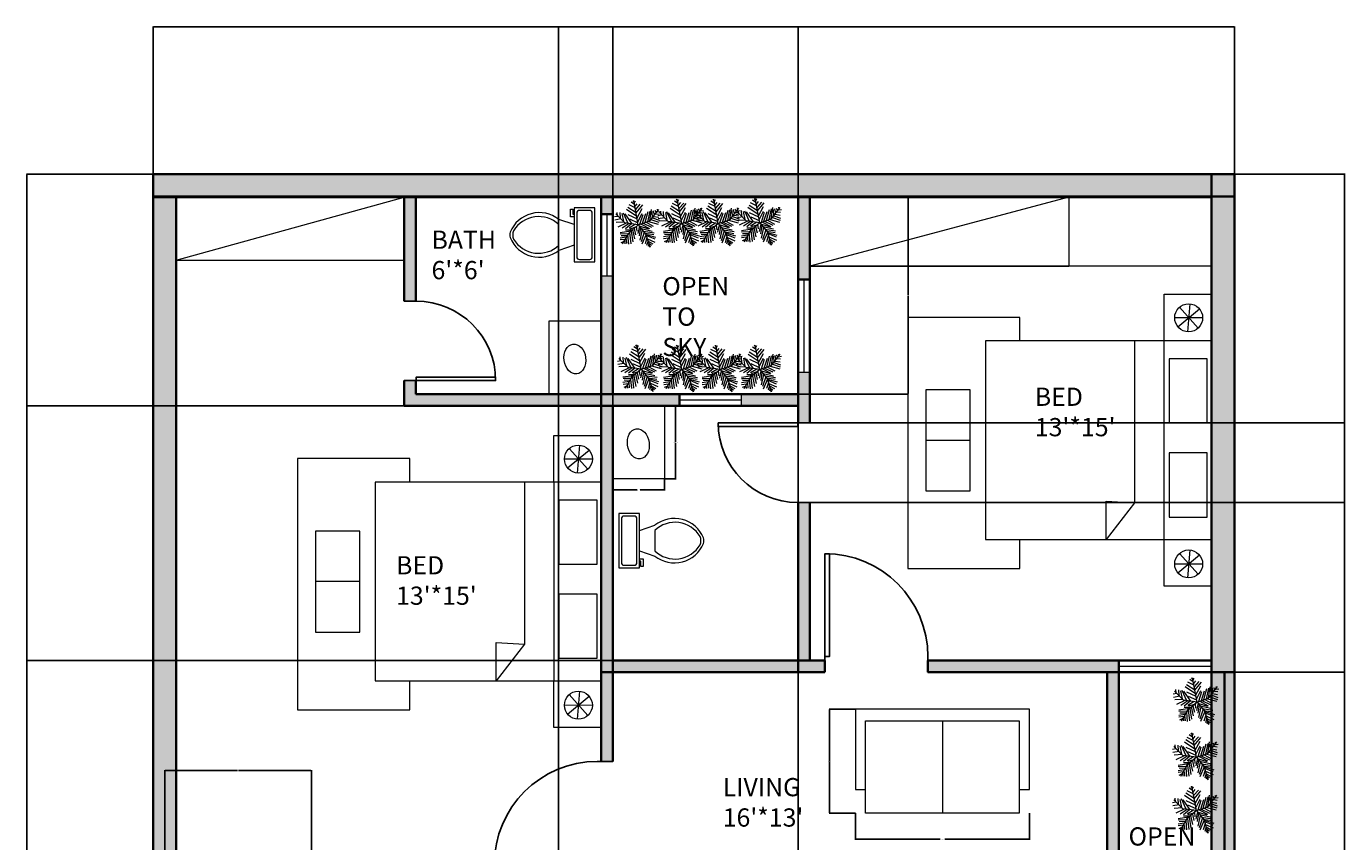
# Model space of a CAD drawing. Units: inches. Extents: x 2119 to 2631, y 2040 to 2935.
# Tile 3 of 3: x 2119 to 2631, y 2618 to 2935. Entities that reach past the tile are written whole.
import ezdxf

# ---------------------------------------------------------------- set-up
doc = ezdxf.new("R2010")
doc.units = ezdxf.units.IN
for name, color, linetype, lineweight in [('A-ANNO-DIMS', 2, 'Continuous', 18), ('A-AREA-IDEN', 7, 'Continuous', 18), ('A-FLOR-CASE', 33, 'Continuous', 18), ('A-FLOR-FIXT', 9, 'Continuous', 18), ('A-WALL-PATT', 252, 'Continuous', 13), ('C-PROP', 7, 'Continuous', 35), ('DOOR', 50, 'Continuous', 25), ('FURNITURE', 220, 'Continuous', 18), ('GRASS', 70, 'Continuous', 13), ('WALL', 180, 'Continuous', 35), ('WINDOW', 130, 'Continuous', 18)]:
    doc.layers.add(name, color=color, linetype=linetype, lineweight=lineweight)
doc.styles.get("Standard").update_dxf_attribs({"font": 'arial.ttf'})
doc.dimstyles.get("Standard").update_dxf_attribs({"dimtxt": 0.18, "dimasz": 0.18, "dimexe": 0.18, "dimexo": 0.0625, "dimgap": 0.09, "dimtad": 0, "dimtih": 1, "dimtoh": 1, "dimdec": 4, "dimzin": 0, "dimdsep": 46, "dimtxsty": 'Standard', "dimcen": 0.09, "dimadec": 0, "dimazin": 0, "dimtfac": 1, "dimtdec": 4, "dimtofl": 0, "dimtmove": 0, "dimatfit": 3, "dimfxl": 1, "dimtolj": 1, "dimtzin": 0, "dimarcsym": 0})

# ---------------------------------------------------------------- blocks, each defined once
blk = doc.blocks.new('*U2')
for p, q in [((0, 0), (0, -6)), ((40, 0), (40, -6))]:
    blk.add_line(p, q)
blk.add_lwpolyline([(0, 0), (0, 40), (1.75, 40), (1.75, 0)], close=True)
blk.add_arc((0, 0), 40, 0, 90)
blk = doc.blocks.new('*U4')
for p, q in [((9.5, -6), (9.5, -2)), ((-10, -8.5), (-8, -8.5)), ((-10, -9.5), (-10, -8.5)), ((-7, -9.5), (-10, -9.5)), ((-8, -8.5), (-8, -8)), ((-7, -8), (-7, -9.5)), ((-4, -8), (-6, -14)), ((4, -8), (6, -14)), ((4, -14), (-4, -14))]:
    blk.add_line(p, q)
blk.add_lwpolyline([(10.5, -8), (10.5, 0), (-10.5, 0), (-10.5, -8)], close=True)
for points in [[(-9.5, -2), (-9.5, -6)], [(8.5, -1), (-8.5, -1)], [(-8.5, -7), (8.5, -7)]]:
    blk.add_lwpolyline(points)
for centre, radius, start, end in [((-8.62, -1.88), 0.884, 81.8699, 188.1301), ((8.62, -1.88), 0.884, 351.8699, 98.1301), ((-8.62, -6.12), 0.884, 171.8699, 278.1301), ((8.62, -6.12), 0.884, 261.8699, 8.1301), ((3.52, -21.58), 12.17, 141.4691, 247.9714), ((4.2, -21.82), 11.33, 136.3677, 238.9468), ((-3.52, -21.58), 12.17, 292.0284, 38.5307), ((-4.2, -21.82), 11.33, 301.053, 43.6321), ((0, -27.88), 4, 245.7318, 294.2682), ((0, -29), 4, 254.8605, 285.1395)]:
    blk.add_arc(centre, radius, start, end)
blk = doc.blocks.new('*U6')
for p, q in [((-3.665, 19.273), (-27.574, 35.527)), ((-5.114, 28.097), (-24.676, 40.636)), ((-7.288, 39.707), (-21.778, 46.673)), ((-8.737, 47.138), (-17.069, 52.711)), ((-10.186, 53.64), (-13.084, 55.962)), ((0, 0), (-10.5, 57)), ((-9.099, 51.782), (-6.563, 55.962)), ((-7.65, 43.423), (-2.578, 49.46)), ((-5.839, 35.992), (4.667, 48.067)), ((-5.114, 27.632), (10.463, 46.673)), ((-2.941, 16.486), (8.652, 37.85)), ((16.259, 5.805), (23.142, 31.348)), ((22.055, 7.198), (27.489, 32.277)), ((27, 9), (48, 36)), ((27.127, 9.056), (31.112, 35.992)), ((35.096, 32.741), (37.27, 22.524)), ((38.719, 34.134), (41.979, 28.561)), ((44.153, 36.456), (45.239, 32.741)), ((-47.498, 19.737), (-55.83, 18.344)), ((-40.615, 13.7), (-55.105, 10.913)), ((-31.5, 4.5), (-52.5, 25.5)), ((-33.37, 6.269), (-52.207, 5.34)), ((-48.585, 21.131), (-49.309, 29.026)), ((-28.299, 3.483), (-47.86, -5.805)), ((-43.513, 28.561), (-42.427, 15.558)), ((-38.442, 26.239), (-34.819, 7.663)), ((-21.416, 3.018), (-38.079, -8.128)), ((-35.544, 28.097), (-24.314, 3.947)), ((0, 0), (-31.5, 4.5)), ((-14.533, 2.09), (-30.834, 25.31)), ((-15.982, 2.09), (-30.11, -9.521)), ((-24.314, 23.917), (-2.941, 13.7)), ((0, 0), (-22.5, -19.5)), ((-6.563, 1.161), (-21.416, -8.128)), ((-20.691, 13.7), (-1.129, 4.876)), ((-1.129, 6.734), (9.014, 26.704)), ((0, 0), (27, 9)), ((0, 0), (18, -22.5)), ((3.942, 1.625), (11.187, 24.381)), ((6.478, 1.625), (26.04, -8.592)), ((10.101, 3.483), (17.708, 26.239)), ((11.187, 3.483), (30.749, -5.805)), ((18.07, 5.805), (35.096, -3.483)), ((24.229, 7.663), (46.688, 1.625)), ((29.662, 12.307), (48.137, 6.269)), ((31.836, 30.883), (32.561, 16.486)), ((33.285, 16.486), (48.862, 10.913)), ((36.183, 19.737), (48.137, 17.88)), ((40.53, 25.775), (48.862, 24.846)), ((43.791, 29.954), (51.036, 30.883)), ((-17.431, -15.094), (-42.789, -18.809)), ((-28.299, -29.026), (-42.789, -31.348)), ((-24.314, -21.596), (-42.427, -22.06)), ((-26.849, -26.24), (-40.253, -25.775)), ((-22.5, -19.5), (-37.5, -45)), ((-15.257, -12.772), (-30.11, -12.772)), ((-29.023, -30.884), (-27.936, -43.887)), ((-25.038, -23.918), (-22.865, -45.281)), ((-20.691, -18.345), (-17.793, -44.352)), ((-6.563, -5.805), (-19.967, -9.985)), ((-17.069, -15.094), (-12.721, -40.172)), ((-13.446, -11.378), (-8.737, -32.741)), ((-9.461, -8.592), (-6.201, -23.453)), ((-4.752, -3.483), (-3.665, -14.629)), ((2.493, -3.019), (-1.491, -20.202)), ((1.769, -2.555), (24.229, -9.521)), ((5.029, -6.27), (2.131, -25.775)), ((9.014, -11.378), (3.58, -35.992)), ((14.085, -16.951), (6.478, -40.172)), ((7.565, -9.056), (32.198, -14.629)), ((18.07, -22.524), (8.289, -45.745)), ((12.274, -15.094), (36.907, -18.809)), ((20.244, -30.419), (15.897, -44.816)), ((16.259, -19.738), (36.183, -22.989)), ((18, -22.5), (27, -52.5)), ((18.433, -22.524), (40.53, -29.026)), ((19.157, -25.311), (38.719, -33.206)), ((-30.834, -34.135), (-42.427, -35.528)), ((-34.457, -39.708), (-40.978, -42.494)), ((-32.646, -36.921), (-31.921, -44.352)), ((22.78, -37.85), (19.519, -48.532)), ((21.331, -32.741), (39.081, -40.636)), ((22.78, -38.314), (34.372, -44.816)), ((24.591, -45.745), (23.142, -50.854)), ((24.591, -43.423), (30.749, -47.603)), ((26.764, -49.925), (28.213, -50.854))]:
    blk.add_line(p, q)
blk = doc.blocks.new('BED-DOUBLE-SUITE')
for p, q in [((-13.02, 5.47), (-4.66, 12.4)), ((-12.38, 13.04), (-5.14, 4.94)), ((-9.21, 3.5), (-8.22, 14.32)), ((-74.36, 9.08), (-117.92, 9.08)), ((-117.92, 9.08), (-117.92, -88.45)), ((-74.36, 0), (-74.36, 9.08)), ((-14.26, 9.02), (-3.4, 8.97)), ((-29.81, 0), (-29.81, -62.95)), ((-18.41, 0), (-18.41, -77.17)), ((-93.69, -38.69), (-110.95, -38.69)), ((-40.83, -77.17), (-40.83, -62.28)), ((-40.83, -62.28), (-29.81, -62.95)), ((-29.81, -62.95), (-40.83, -77.17)), ((-74.36, -88.45), (-74.36, -77.17)), ((-9.21, -92.12), (-8.22, -81.31)), ((-14.26, -86.6), (-3.4, -86.65)), ((-13.02, -90.15), (-4.66, -83.22)), ((-12.38, -82.59), (-5.14, -90.68)), ((-117.92, -88.45), (-74.36, -88.45))]:
    blk.add_line(p, q)
for points in [[(0, 0), (-18.39, 0), (-18.39, 18.13), (0, 18.13)], [(0, 0), (-87.71, 0), (-87.71, -77.17), (0, -77.17)], [(-1.58, -7.03), (-16.39, -7.03), (-16.39, -31.92), (-1.58, -31.92)], [(-93.69, -19.1), (-110.95, -19.1), (-110.95, -58.28), (-93.69, -58.28)], [(-1.58, -43.58), (-16.39, -43.58), (-16.39, -68.47), (-1.58, -68.47)], [(0, -95.3), (-18.39, -95.3), (-18.39, -77.17), (0, -77.17)]]:
    blk.add_lwpolyline(points, close=True)
for centre in [(-8.83, 8.92), (-8.83, -86.7)]:
    blk.add_circle(centre, 5.43)
blk = doc.blocks.new('SOFA-2-SEAT')
for p, q in [((-9.19, 63.72), (-40.39, 63.72)), ((-40.39, 63.72), (-40.39, -3.87)), ((-9.19, 59.66), (-9.19, 63.72)), ((-35.92, 29.83), (0, 29.83)), ((-9.19, -3.87), (-9.19, 0)), ((-40.39, -3.87), (-9.19, -3.87))]:
    blk.add_line(p, q)
blk.add_lwpolyline([(0, 0), (-35.92, 0), (-35.92, 59.66), (0, 59.66)], close=True)
blk = doc.blocks.new('BASIN-VANITY')
blk.add_lwpolyline([(0, 0), (-20.15, 0), (-20.15, 28.46), (0, 28.46)], close=True)
blk.add_ellipse((-10.21, 13.63), major_axis=(0.77, -5.8), ratio=0.722636)
blk = doc.blocks.new('*D14')
at = {"layer": 'A-ANNO-DIMS', "color": 0, "lineweight": -2, "transparency": 16777216}
for p, q in [((2441.07, 2629.04), (2441.07, 2618.79)), ((2508.66, 2629.04), (2508.66, 2618.79)), ((2441.25, 2618.97), (2473.96, 2618.97)), ((2508.48, 2618.97), (2475.77, 2618.97))]:
    blk.add_line(p, q, dxfattribs=at)
at = {"layer": 'A-ANNO-DIMS', "color": 0, "lineweight": 100, "transparency": 16777216}
for points in [[(2441.25, 2619), (2441.25, 2618.94), (2441.07, 2618.97)], [(2508.48, 2619), (2508.48, 2618.94), (2508.66, 2618.97)]]:
    blk.add_solid(points, dxfattribs=at)
at = {"layer": 'Defpoints', "color": 0, "lineweight": 100, "transparency": 16777216}
for p in [(2441.07, 2629.11), (2508.66, 2629.11), (2508.66, 2618.97)]:
    blk.add_point(p, dxfattribs=at)
at = {"layer": 'A-ANNO-DIMS', "color": 0, "transparency": 16777216, "insert": (2474.87, 2618.97), "char_height": 0.18, "attachment_point": 5}
blk.add_mtext('\\A1;SOFA 68 TYP.', dxfattribs=at)
blk = doc.blocks.new('*D15')
at = {"layer": 'A-ANNO-DIMS', "color": 0, "lineweight": -2, "transparency": 16777216}
for p, q in [((2441.01, 2669.5), (2430.76, 2669.5)), ((2430.94, 2669.32), (2430.94, 2649.48)), ((2430.94, 2629.29), (2430.94, 2649.12)), ((2441.01, 2629.11), (2430.76, 2629.11))]:
    blk.add_line(p, q, dxfattribs=at)
at = {"layer": 'A-ANNO-DIMS', "color": 0, "lineweight": 100, "transparency": 16777216}
for points in [[(2430.91, 2669.32), (2430.97, 2669.32), (2430.94, 2669.5)], [(2430.91, 2629.29), (2430.97, 2629.29), (2430.94, 2629.11)]]:
    blk.add_solid(points, dxfattribs=at)
at = {"layer": 'Defpoints', "color": 0, "lineweight": 100, "transparency": 16777216}
for p in [(2441.07, 2669.5), (2430.94, 2629.11), (2441.07, 2629.11)]:
    blk.add_point(p, dxfattribs=at)
at = {"layer": 'A-ANNO-DIMS', "color": 0, "transparency": 16777216, "insert": (2430.94, 2649.3), "char_height": 0.18, "attachment_point": 5}
blk.add_mtext('\\A1;40 TYP.', dxfattribs=at)
blk = doc.blocks.new('*D16')
at = {"layer": 'A-ANNO-DIMS', "color": 0, "lineweight": -2, "transparency": 16777216}
for p, q in [((2366.96, 2787.4), (2371.35, 2787.4)), ((2371.17, 2787.22), (2371.17, 2773.35)), ((2371.17, 2759.12), (2371.17, 2772.99)), ((2366.96, 2758.94), (2371.35, 2758.94))]:
    blk.add_line(p, q, dxfattribs=at)
at = {"layer": 'A-ANNO-DIMS', "color": 0, "lineweight": 100, "transparency": 16777216}
for points in [[(2371.14, 2787.22), (2371.2, 2787.22), (2371.17, 2787.4)], [(2371.14, 2759.12), (2371.2, 2759.12), (2371.17, 2758.94)]]:
    blk.add_solid(points, dxfattribs=at)
at = {"layer": 'Defpoints', "color": 0, "lineweight": 100, "transparency": 16777216}
for p in [(2366.9, 2787.4), (2371.17, 2787.4), (2366.9, 2758.94)]:
    blk.add_point(p, dxfattribs=at)
at = {"layer": 'A-ANNO-DIMS', "color": 0, "transparency": 16777216, "insert": (2371.17, 2773.17), "char_height": 0.18, "attachment_point": 5}
blk.add_mtext('\\A1;VANITY 28 TYP.', dxfattribs=at)
blk = doc.blocks.new('*D17')
at = {"layer": 'A-ANNO-DIMS', "color": 0, "lineweight": -2, "transparency": 16777216}
for p, q in [((2346.75, 2758.88), (2346.75, 2754.49)), ((2366.9, 2758.88), (2366.9, 2754.49)), ((2346.93, 2754.67), (2356.3, 2754.67)), ((2366.72, 2754.67), (2357.36, 2754.67))]:
    blk.add_line(p, q, dxfattribs=at)
at = {"layer": 'A-ANNO-DIMS', "color": 0, "lineweight": 100, "transparency": 16777216}
for points in [[(2346.93, 2754.7), (2346.93, 2754.64), (2346.75, 2754.67)], [(2366.72, 2754.7), (2366.72, 2754.64), (2366.9, 2754.67)]]:
    blk.add_solid(points, dxfattribs=at)
at = {"layer": 'Defpoints', "color": 0, "lineweight": 100, "transparency": 16777216}
for p in [(2346.75, 2758.94), (2366.9, 2758.94), (2366.9, 2754.67)]:
    blk.add_point(p, dxfattribs=at)
at = {"layer": 'A-ANNO-DIMS', "color": 0, "transparency": 16777216, "insert": (2356.83, 2754.67), "char_height": 0.18, "attachment_point": 5}
blk.add_mtext('\\A1;20 TYP.', dxfattribs=at)
blk = doc.blocks.new('*D18')
at = {"layer": 'A-ANNO-DIMS', "color": 0, "lineweight": -2, "transparency": 16777216}
for p, q in [((2168.25, 2877.46), (2168.25, 2934.76)), ((2168.43, 2934.58), (2377.96, 2934.58)), ((2588.07, 2934.58), (2378.55, 2934.58)), ((2588.25, 2877.46), (2588.25, 2934.76))]:
    blk.add_line(p, q, dxfattribs=at)
at = {"layer": 'A-ANNO-DIMS', "color": 0, "lineweight": 100, "transparency": 16777216}
for points in [[(2168.43, 2934.61), (2168.43, 2934.55), (2168.25, 2934.58)], [(2588.07, 2934.61), (2588.07, 2934.55), (2588.25, 2934.58)]]:
    blk.add_solid(points, dxfattribs=at)
at = {"layer": 'Defpoints', "color": 0, "lineweight": 100, "transparency": 16777216}
for p in [(2588.25, 2934.58), (2168.25, 2877.4), (2588.25, 2877.4)]:
    blk.add_point(p, dxfattribs=at)
at = {"layer": 'A-ANNO-DIMS', "color": 0, "transparency": 16777216, "insert": (2378.25, 2934.58), "char_height": 0.18, "attachment_point": 5}
blk.add_mtext('\\A1;420', dxfattribs=at)
blk = doc.blocks.new('*D19')
at = {"layer": 'A-ANNO-DIMS', "color": 0, "lineweight": -2, "transparency": 16777216}
for p, q in [((2168.19, 2877.4), (2119.07, 2877.4)), ((2119.25, 2877.22), (2119.25, 2487.58)), ((2119.25, 2097.58), (2119.25, 2487.22)), ((2168.19, 2097.4), (2119.07, 2097.4))]:
    blk.add_line(p, q, dxfattribs=at)
at = {"layer": 'A-ANNO-DIMS', "color": 0, "lineweight": 100, "transparency": 16777216}
for points in [[(2119.22, 2877.22), (2119.28, 2877.22), (2119.25, 2877.4)], [(2119.22, 2097.58), (2119.28, 2097.58), (2119.25, 2097.4)]]:
    blk.add_solid(points, dxfattribs=at)
at = {"layer": 'Defpoints', "color": 0, "lineweight": 100, "transparency": 16777216}
for p in [(2119.25, 2877.4), (2168.25, 2877.4), (2168.25, 2097.4)]:
    blk.add_point(p, dxfattribs=at)
at = {"layer": 'A-ANNO-DIMS', "color": 0, "transparency": 16777216, "insert": (2119.25, 2487.4), "char_height": 0.18, "attachment_point": 5}
blk.add_mtext('\\A1;780', dxfattribs=at)
blk = doc.blocks.new('*D21')
at = {"layer": 'A-ANNO-DIMS', "color": 0, "lineweight": -2, "transparency": 16777216}
for p, q in [((2325.75, 2175.46), (2325.75, 2934.76)), ((2325.93, 2934.58), (2372.04, 2934.58)), ((2418.57, 2934.58), (2372.47, 2934.58)), ((2418.75, 2175.46), (2418.75, 2934.76))]:
    blk.add_line(p, q, dxfattribs=at)
at = {"layer": 'A-ANNO-DIMS', "color": 0, "lineweight": 100, "transparency": 16777216}
for points in [[(2325.93, 2934.61), (2325.93, 2934.55), (2325.75, 2934.58)], [(2418.57, 2934.61), (2418.57, 2934.55), (2418.75, 2934.58)]]:
    blk.add_solid(points, dxfattribs=at)
at = {"layer": 'Defpoints', "color": 0, "lineweight": 100, "transparency": 16777216}
for p in [(2418.75, 2934.58), (2325.75, 2175.4), (2418.75, 2175.4)]:
    blk.add_point(p, dxfattribs=at)
at = {"layer": 'A-ANNO-DIMS', "color": 0, "transparency": 16777216, "insert": (2372.25, 2934.58), "char_height": 0.18, "attachment_point": 5}
blk.add_mtext('\\A1;93', dxfattribs=at)
blk = doc.blocks.new('*D25')
at = {"layer": 'A-ANNO-DIMS', "color": 0, "lineweight": -2, "transparency": 16777216}
for p, q in [((2588.32, 2683.9), (2631.18, 2683.9)), ((2631, 2683.72), (2631, 2606.21)), ((2631, 2528.34), (2631, 2605.85)), ((2588.32, 2528.16), (2631.18, 2528.16))]:
    blk.add_line(p, q, dxfattribs=at)
at = {"layer": 'A-ANNO-DIMS', "color": 0, "lineweight": 100, "transparency": 16777216}
for points in [[(2630.97, 2683.72), (2631.03, 2683.72), (2631, 2683.9)], [(2630.97, 2528.34), (2631.03, 2528.34), (2631, 2528.16)]]:
    blk.add_solid(points, dxfattribs=at)
at = {"layer": 'Defpoints', "color": 0, "lineweight": 100, "transparency": 16777216}
for p in [(2588.25, 2683.9), (2631, 2683.9), (2588.25, 2528.16)]:
    blk.add_point(p, dxfattribs=at)
at = {"layer": 'A-ANNO-DIMS', "color": 0, "transparency": 16777216, "insert": (2631, 2606.03), "char_height": 0.18, "attachment_point": 5}
blk.add_mtext('\\A1;155.74', dxfattribs=at)
blk = doc.blocks.new('*D26')
at = {"layer": 'A-ANNO-DIMS', "color": 0, "lineweight": -2, "transparency": 16777216}
for p, q in [((2588.32, 2877.4), (2631.18, 2877.4)), ((2631, 2877.22), (2631, 2780.83)), ((2631, 2684.08), (2631, 2780.47)), ((2588.32, 2683.9), (2631.18, 2683.9))]:
    blk.add_line(p, q, dxfattribs=at)
at = {"layer": 'A-ANNO-DIMS', "color": 0, "lineweight": 100, "transparency": 16777216}
for points in [[(2630.97, 2877.22), (2631.03, 2877.22), (2631, 2877.4)], [(2630.97, 2684.08), (2631.03, 2684.08), (2631, 2683.9)]]:
    blk.add_solid(points, dxfattribs=at)
at = {"layer": 'Defpoints', "color": 0, "lineweight": 100, "transparency": 16777216}
for p in [(2588.25, 2877.4), (2631, 2877.4), (2588.25, 2683.9)]:
    blk.add_point(p, dxfattribs=at)
at = {"layer": 'A-ANNO-DIMS', "color": 0, "transparency": 16777216, "insert": (2631, 2780.65), "char_height": 0.18, "attachment_point": 5}
blk.add_mtext('\\A1;193.5', dxfattribs=at)
blk = doc.blocks.new('*D27')
at = {"layer": 'A-ANNO-DIMS', "color": 0, "lineweight": -2, "transparency": 16777216}
for p, q in [((2346.75, 2688.46), (2346.75, 2934.76)), ((2346.93, 2934.58), (2382.54, 2934.58)), ((2418.57, 2934.58), (2382.97, 2934.58)), ((2418.75, 2688.46), (2418.75, 2934.76))]:
    blk.add_line(p, q, dxfattribs=at)
at = {"layer": 'A-ANNO-DIMS', "color": 0, "lineweight": 100, "transparency": 16777216}
for points in [[(2346.93, 2934.61), (2346.93, 2934.55), (2346.75, 2934.58)], [(2418.57, 2934.61), (2418.57, 2934.55), (2418.75, 2934.58)]]:
    blk.add_solid(points, dxfattribs=at)
at = {"layer": 'Defpoints', "color": 0, "lineweight": 100, "transparency": 16777216}
for p in [(2418.75, 2934.58), (2346.75, 2688.4), (2418.75, 2688.4)]:
    blk.add_point(p, dxfattribs=at)
at = {"layer": 'A-ANNO-DIMS', "color": 0, "transparency": 16777216, "insert": (2382.75, 2934.58), "char_height": 0.18, "attachment_point": 5}
blk.add_mtext('\\A1;72', dxfattribs=at)
blk = doc.blocks.new('*D28')
at = {"layer": 'A-ANNO-DIMS', "color": 0, "lineweight": -2, "transparency": 16777216}
for p, q in [((2418.69, 2787.4), (2119.07, 2787.4)), ((2119.25, 2787.22), (2119.25, 2738.08)), ((2119.25, 2688.58), (2119.25, 2737.72)), ((2418.69, 2688.4), (2119.07, 2688.4))]:
    blk.add_line(p, q, dxfattribs=at)
at = {"layer": 'A-ANNO-DIMS', "color": 0, "lineweight": 100, "transparency": 16777216}
for points in [[(2119.22, 2787.22), (2119.28, 2787.22), (2119.25, 2787.4)], [(2119.22, 2688.58), (2119.28, 2688.58), (2119.25, 2688.4)]]:
    blk.add_solid(points, dxfattribs=at)
at = {"layer": 'Defpoints', "color": 0, "lineweight": 100, "transparency": 16777216}
for p in [(2119.25, 2787.4), (2418.75, 2787.4), (2418.75, 2688.4)]:
    blk.add_point(p, dxfattribs=at)
at = {"layer": 'A-ANNO-DIMS', "color": 0, "transparency": 16777216, "insert": (2119.25, 2737.9), "char_height": 0.18, "attachment_point": 5}
blk.add_mtext('\\A1;99', dxfattribs=at)
blk = doc.blocks.new('*D29')
at = {"layer": 'A-ANNO-DIMS', "color": 0, "lineweight": -2, "transparency": 16777216}
for p, q in [((2423.32, 2780.71), (2631.18, 2780.71)), ((2631, 2780.53), (2631, 2765.45)), ((2631, 2749.99), (2631, 2765.08)), ((2423.32, 2749.81), (2631.18, 2749.81))]:
    blk.add_line(p, q, dxfattribs=at)
at = {"layer": 'A-ANNO-DIMS', "color": 0, "lineweight": 100, "transparency": 16777216}
for points in [[(2630.97, 2780.53), (2631.03, 2780.53), (2631, 2780.71)], [(2630.97, 2749.99), (2631.03, 2749.99), (2631, 2749.81)]]:
    blk.add_solid(points, dxfattribs=at)
at = {"layer": 'Defpoints', "color": 0, "lineweight": 100, "transparency": 16777216}
for p in [(2423.25, 2780.71), (2631, 2780.71), (2423.25, 2749.81)]:
    blk.add_point(p, dxfattribs=at)
at = {"layer": 'A-ANNO-DIMS', "color": 0, "transparency": 16777216, "insert": (2631, 2765.26), "char_height": 0.18, "attachment_point": 5}
blk.add_mtext('\\A1;30.897', dxfattribs=at)
blk = doc.blocks.new('*D30')
at = {"layer": 'A-ANNO-DIMS', "color": 0, "lineweight": -2, "transparency": 16777216}
for p, q in [((2172.75, 2602.96), (2172.75, 2645.83)), ((2172.93, 2645.65), (2201.04, 2645.65)), ((2229.57, 2645.65), (2201.47, 2645.65)), ((2229.75, 2602.96), (2229.75, 2645.83))]:
    blk.add_line(p, q, dxfattribs=at)
at = {"layer": 'A-ANNO-DIMS', "color": 0, "lineweight": 100, "transparency": 16777216}
for points in [[(2172.93, 2645.68), (2172.93, 2645.62), (2172.75, 2645.65)], [(2229.57, 2645.68), (2229.57, 2645.62), (2229.75, 2645.65)]]:
    blk.add_solid(points, dxfattribs=at)
at = {"layer": 'Defpoints', "color": 0, "lineweight": 100, "transparency": 16777216}
for p in [(2229.75, 2645.65), (2172.75, 2602.9), (2229.75, 2602.9)]:
    blk.add_point(p, dxfattribs=at)
at = {"layer": 'A-ANNO-DIMS', "color": 0, "transparency": 16777216, "insert": (2201.25, 2645.65), "char_height": 0.18, "attachment_point": 5}
blk.add_mtext('\\A1;57', dxfattribs=at)
blk = doc.blocks.new('*D31')
at = {"layer": 'A-ANNO-DIMS', "color": 0, "lineweight": -2, "transparency": 16777216}
for p, q in [((2543.25, 2683.84), (2543.25, 2054.47)), ((2579.25, 2683.84), (2579.25, 2054.47)), ((2543.43, 2054.65), (2561.04, 2054.65)), ((2579.07, 2054.65), (2561.47, 2054.65))]:
    blk.add_line(p, q, dxfattribs=at)
at = {"layer": 'A-ANNO-DIMS', "color": 0, "lineweight": 100, "transparency": 16777216}
for points in [[(2543.43, 2054.68), (2543.43, 2054.62), (2543.25, 2054.65)], [(2579.07, 2054.68), (2579.07, 2054.62), (2579.25, 2054.65)]]:
    blk.add_solid(points, dxfattribs=at)
at = {"layer": 'Defpoints', "color": 0, "lineweight": 100, "transparency": 16777216}
for p in [(2543.25, 2683.9), (2579.25, 2683.9), (2579.25, 2054.65)]:
    blk.add_point(p, dxfattribs=at)
at = {"layer": 'A-ANNO-DIMS', "color": 0, "transparency": 16777216, "insert": (2561.25, 2054.65), "char_height": 0.18, "attachment_point": 5}
blk.add_mtext('\\A1;36', dxfattribs=at)
blk = doc.blocks.new('*D32')
at = {"layer": 'A-ANNO-DIMS', "color": 0, "lineweight": -2, "transparency": 16777216}
for p, q in [((2418.82, 2868.4), (2461.68, 2868.4)), ((2461.5, 2868.22), (2461.5, 2830.33)), ((2461.5, 2792.08), (2461.5, 2829.97)), ((2418.82, 2791.9), (2461.68, 2791.9))]:
    blk.add_line(p, q, dxfattribs=at)
at = {"layer": 'A-ANNO-DIMS', "color": 0, "lineweight": 100, "transparency": 16777216}
for points in [[(2461.47, 2868.22), (2461.53, 2868.22), (2461.5, 2868.4)], [(2461.47, 2792.08), (2461.53, 2792.08), (2461.5, 2791.9)]]:
    blk.add_solid(points, dxfattribs=at)
at = {"layer": 'Defpoints', "color": 0, "lineweight": 100, "transparency": 16777216}
for p in [(2418.75, 2868.4), (2418.75, 2791.9), (2461.5, 2791.9)]:
    blk.add_point(p, dxfattribs=at)
at = {"layer": 'A-ANNO-DIMS', "color": 0, "transparency": 16777216, "insert": (2461.5, 2830.15), "char_height": 0.18, "attachment_point": 5}
blk.add_mtext('\\A1;76.5', dxfattribs=at)

msp = doc.modelspace()

# ---------------------------------------------------------------- hatches: boundary and pattern name
at = {"layer": 'A-WALL-PATT'}
h = msp.add_hatch(color=256, dxfattribs=at)
h.dxf.hatch_style = 1
h.paths.add_polyline_path([(2177.2549, 2868.3983), (2168.2549, 2868.3983), (2168.2549, 2602.8983), (2177.2549, 2602.8983)])
h.paths.add_polyline_path([(2588.2549, 2877.3983), (2579.2549, 2877.3983), (2579.2549, 2868.6805), (2588.2549, 2868.6805)])
h.paths.add_polyline_path([(2579.2549, 2877.3983), (2168.2549, 2877.3983), (2168.2549, 2868.6805), (2579.2549, 2868.6805)])
h.paths.add_polyline_path([(2588.2549, 2868.6805), (2579.2549, 2868.6805), (2579.2549, 2166.3983), (2588.2549, 2166.3983)])
h = msp.add_hatch(color=256, dxfattribs=at)
h.dxf.hatch_style = 1
h.paths.add_polyline_path([(2270.2549, 2868.3983), (2265.7549, 2868.3983), (2265.7549, 2843.8762), (2265.7549, 2828.0189), (2270.2549, 2828.0189)])
h.paths.add_polyline_path([(2342.2549, 2791.8983), (2322.1084, 2791.8983), (2270.2549, 2791.8983), (2270.2549, 2797.1221), (2265.7549, 2797.1221), (2265.7549, 2787.3983), (2342.2549, 2787.3983)])
h = msp.add_hatch(color=256, dxfattribs=at)
h.dxf.hatch_style = 1
h.paths.add_polyline_path([(2423.2549, 2868.3983), (2418.7549, 2868.3983), (2418.7549, 2836.4443), (2423.2549, 2836.4443)])
h.paths.add_polyline_path([(2346.7549, 2868.3983), (2342.2549, 2868.3983), (2342.2549, 2861.8041), (2346.7549, 2861.8041)])
h = msp.add_hatch(color=256, dxfattribs=at)
h.dxf.hatch_style = 1
h.paths.add_polyline_path([(2346.7549, 2683.8983), (2342.2549, 2683.8983), (2342.2549, 2662.4397), (2342.2549, 2649.1862), (2346.7549, 2649.1862)])
h.paths.add_polyline_path([(2346.7549, 2787.3983), (2342.2549, 2787.3983), (2342.2549, 2683.8983), (2346.7549, 2683.8983), (2346.7549, 2688.3983)])
h.paths.add_polyline_path([(2418.7549, 2688.3983), (2346.7549, 2688.3983), (2346.7549, 2683.8983), (2418.7549, 2683.8983)])
h.paths.add_polyline_path([(2429.1646, 2688.3983), (2418.7549, 2688.3983), (2418.7549, 2683.8983), (2429.1646, 2683.8983)])
h.paths.add_polyline_path([(2423.2549, 2749.8147), (2418.7549, 2749.8147), (2418.7549, 2688.3983), (2423.2549, 2688.3983)])
h.paths.add_polyline_path([(2543.2549, 2688.3983), (2469.1646, 2688.3983), (2469.1646, 2683.8983), (2543.2549, 2683.8983)])
h.paths.add_polyline_path([(2423.2549, 2800.4443), (2418.7549, 2800.4443), (2418.7549, 2780.7115), (2423.2549, 2780.7115)])
h.paths.add_polyline_path([(2346.7549, 2837.8041), (2342.2549, 2837.8041), (2342.2549, 2791.8983), (2346.7549, 2791.8983)])
h.paths.add_polyline_path([(2372.6689, 2791.8983), (2342.2549, 2791.8983), (2342.2549, 2787.3983), (2346.7549, 2787.3983), (2372.6689, 2787.3983)])
h.paths.add_polyline_path([(2418.7549, 2791.8983), (2396.6689, 2791.8983), (2396.6689, 2787.3983), (2418.7549, 2787.3983)])
h = msp.add_hatch(color=256, dxfattribs=at)
h.dxf.hatch_style = 1
h.paths.add_polyline_path([(2543.2549, 2683.8983), (2538.7549, 2683.8983), (2538.7549, 2523.3983), (2543.2549, 2523.3983)])

# ---------------------------------------------------------------- linework, layer by layer
at = {"layer": 'A-FLOR-CASE'}
for p, q in [((2177.2549, 2843.8762), (2265.7549, 2868.3983)), ((2523.8469, 2868.3983), (2423.2549, 2841.6228)), ((2523.8469, 2868.3983), (2523.8469, 2841.6228)), ((2423.2549, 2841.6228), (2523.8469, 2841.6228))]:
    msp.add_line(p, q, dxfattribs=at)
for points in [[(2265.7549, 2868.3983), (2177.2549, 2868.3983), (2177.2549, 2843.8762), (2265.7549, 2843.8762)], [(2423.2549, 2868.3983), (2579.2549, 2868.3983), (2579.2549, 2841.6228), (2423.2549, 2841.6228)]]:
    msp.add_lwpolyline(points, close=True, dxfattribs=at)
at = {"layer": 'A-FLOR-FIXT'}
msp.add_lwpolyline([(2342.2549, 2791.8983), (2322.1084, 2791.8983), (2322.1084, 2820.3551), (2342.2549, 2820.3551)], close=True, dxfattribs=at)
msp.add_ellipse((2332.0453, 2805.5326), major_axis=(0.7738, -5.7989), ratio=0.72263565, dxfattribs=at)
at = {"layer": 'C-PROP'}
msp.add_lwpolyline([(2168.2549, 2097.3983), (2588.2549, 2097.3983), (2588.2549, 2877.3983), (2168.2549, 2877.3983)], close=True, dxfattribs=at)
at = {"layer": 'WALL'}
for p, q in [((2265.7549, 2868.3983), (2265.7549, 2828.0189)), ((2342.2549, 2868.3983), (2270.2549, 2868.3983)), ((2270.2549, 2868.3983), (2270.2549, 2828.0189)), ((2342.2549, 2791.8983), (2342.2549, 2868.3983)), ((2346.7549, 2791.8983), (2346.7549, 2868.3983)), ((2418.7549, 2868.3983), (2418.7549, 2780.7115)), ((2579.2549, 2868.3983), (2423.2549, 2868.3983)), ((2423.2549, 2868.3983), (2423.2549, 2780.7115)), ((2579.2549, 2833.3004), (2579.2549, 2710.1197)), ((2265.7549, 2797.1221), (2265.7549, 2787.3983)), ((2270.2549, 2797.1221), (2270.2549, 2791.8983)), ((2265.7549, 2787.3983), (2342.2549, 2787.3983)), ((2270.2549, 2791.8983), (2342.2549, 2791.8983)), ((2342.2549, 2683.8983), (2342.2549, 2791.8983)), ((2342.2549, 2791.8983), (2418.7549, 2791.8983)), ((2342.2549, 2787.3983), (2342.2549, 2649.1862)), ((2346.7549, 2688.3983), (2346.7549, 2787.3983)), ((2346.7549, 2787.3983), (2418.7549, 2787.3983)), ((2346.7549, 2787.3983), (2346.7549, 2649.1862)), ((2342.2549, 2775.8749), (2342.2549, 2662.4397)), ((2418.7549, 2749.8147), (2418.7549, 2683.8983)), ((2423.2549, 2749.8147), (2423.2549, 2688.3983)), ((2418.7549, 2688.3983), (2346.7549, 2688.3983)), ((2423.2549, 2688.3983), (2429.1646, 2688.3983)), ((2423.2549, 2688.3983), (2429.1646, 2688.3983)), ((2469.1646, 2688.3983), (2579.2549, 2688.3983)), ((2418.7549, 2683.8983), (2342.2549, 2683.8983)), ((2346.7549, 2683.8983), (2429.1646, 2683.8983)), ((2418.7549, 2683.8983), (2429.1646, 2683.8983)), ((2469.1646, 2683.8983), (2538.7549, 2683.8983)), ((2469.1646, 2683.8983), (2579.2549, 2683.8983)), ((2538.7549, 2683.8983), (2538.7549, 2527.8983)), ((2543.2549, 2683.8983), (2543.2549, 2523.3983)), ((2579.2549, 2683.8983), (2588.2549, 2683.8983)), ((2584.2794, 2683.8983), (2584.2794, 2528.1615))]:
    msp.add_line(p, q, dxfattribs=at)
for points in [[(2168.2549, 2877.3983), (2588.2549, 2877.3983), (2588.2549, 2868.6805), (2168.2549, 2868.6805)], [(2588.2549, 2877.3983), (2579.2549, 2877.3983), (2579.2549, 2166.3983), (2588.2549, 2166.3983)], [(2168.2549, 2602.8983), (2177.2549, 2602.8983), (2177.2549, 2868.3983), (2168.2549, 2868.3983)], [(2342.2549, 2868.3983), (2346.7549, 2868.3983), (2346.7549, 2861.8041), (2342.2549, 2861.8041)], [(2418.7549, 2868.3983), (2423.2549, 2868.3983), (2423.2549, 2836.4443), (2418.7549, 2836.4443)], [(2342.2549, 2791.8983), (2372.6689, 2791.8983), (2372.6689, 2787.3983), (2342.2549, 2787.3983)], [(2342.2549, 2787.3983), (2346.7549, 2787.3983), (2346.7549, 2683.8983), (2342.2549, 2683.8983)], [(2429.1646, 2683.8983), (2346.7549, 2683.8983), (2346.7549, 2688.3983), (2429.1646, 2688.3983)], [(2543.2549, 2688.3983), (2469.1646, 2688.3983), (2469.1646, 2683.8983), (2543.2549, 2683.8983)], [(2538.7549, 2683.8983), (2543.2549, 2683.8983), (2543.2549, 2523.3983), (2538.7549, 2523.3983)]]:
    msp.add_lwpolyline(points, close=True, dxfattribs=at)
for points in [[(2342.2549, 2868.3983), (2177.2549, 2868.3983), (2177.2549, 2602.8983)], [(2418.7549, 2868.3983), (2346.7549, 2868.3983)], [(2579.2549, 2683.8983), (2579.2549, 2868.3983), (2423.2549, 2868.3983)]]:
    msp.add_lwpolyline(points, dxfattribs=at)
at = {"layer": 'WINDOW'}
for p, q in [((2342.2549, 2861.8041), (2346.7549, 2861.8041)), ((2344.5049, 2861.8041), (2344.5049, 2837.8041)), ((2342.2549, 2837.8041), (2346.7549, 2837.8041)), ((2418.7549, 2836.4443), (2423.2549, 2836.4443)), ((2421.0049, 2836.4443), (2421.0049, 2800.4443)), ((2418.7549, 2800.4443), (2423.2549, 2800.4443)), ((2372.6689, 2791.8983), (2372.6689, 2787.3983)), ((2372.6689, 2789.6483), (2396.6689, 2789.6483)), ((2396.6689, 2791.8983), (2396.6689, 2787.3983)), ((2543.2549, 2683.8983), (2543.2549, 2688.3983)), ((2543.2549, 2688.3983), (2579.2549, 2688.3983)), ((2543.2549, 2686.1483), (2579.2549, 2686.1483))]:
    msp.add_line(p, q, dxfattribs=at)
msp.add_lwpolyline([(2543.2549, 2683.8983), (2579.2549, 2683.8983), (2579.2549, 2688.3983), (2543.2549, 2688.3983)], close=True, dxfattribs=at)

# ---------------------------------------------------------------- block references
at = {"layer": 'A-FLOR-FIXT'}
for p, rotation in [((2339.8024, 2853.7456), 270), ((2349.1305, 2734.9666), 89.99999999999999)]:
    msp.add_blockref('*U4', p, dxfattribs=dict(at, rotation=rotation))
msp.add_blockref('BASIN-VANITY', (2366.9014, 2758.9415), dxfattribs=at)
at = {"layer": 'DOOR', "xscale": -0.7724210789723547, "yscale": 0.7724210789723547, "zscale": 0.7724210789723547}
for p, rotation in [((2270.3894, 2797.1221), 270), ((2418.6204, 2780.7115), 90)]:
    msp.add_blockref('*U2', p, dxfattribs=dict(at, rotation=rotation))
at = {"layer": 'DOOR'}
msp.add_blockref('*U2', (2429.1646, 2689.8983), dxfattribs=at)
at = {"layer": 'DOOR', "rotation": 89.99999999999999}
msp.add_blockref('*U2', (2340.7549, 2609.1862), dxfattribs=at)
at = {"layer": 'FURNITURE'}
for p in [(2579.2549, 2812.6252), (2342.2549, 2757.741)]:
    msp.add_blockref('BED-DOUBLE-SUITE', p, dxfattribs=at)
at = {"layer": 'FURNITURE', "rotation": 270.0000000000005}
msp.add_blockref('SOFA-2-SEAT', (2444.9403, 2629.106), dxfattribs=at)
at = {"layer": 'GRASS', "xscale": 0.1657890412075336, "yscale": 0.1657890412075336, "zscale": 0.1657890412075336}
for p in [(2356.6915, 2857.6818), (2373.5702, 2858.1591), (2387.742, 2858.1591), (2403.8246, 2858.4773), (2357.8323, 2801.5556), (2373.5744, 2801.456), (2388.5194, 2801.456), (2403.863, 2801.456), (2573.677, 2672.2749), (2573.4211, 2650.7931), (2573.4211, 2630.0785)]:
    msp.add_blockref('*U6', p, dxfattribs=at)

# ---------------------------------------------------------------- texts
at = {"layer": 'A-AREA-IDEN', "attachment_point": 1}
for s, insert, char_height in [("BATH\\P6'*6'", (2276.3803, 2855.4179), 7.08052), ('OPEN TO  SKY', (2366.0194, 2837.3549), 7.080524), ("BED\\P13'*15'", (2510.6846, 2794.4079), 7.08052), ("BED\\P13'*15'", (2262.6051, 2728.932), 7.08052), ("LIVING\\P16'*13'", (2389.4664, 2642.7543), 7.08052), ('OPEN TO SKY', (2547.0829, 2623.5978), 7.080524)]:
    msp.add_mtext_dynamic_manual_height_columns(s, width=32.794808, gutter_width=35.4026, heights=[0], dxfattribs=dict(at, insert=insert, char_height=char_height))

# ---------------------------------------------------------------- dimensions: what is measured, and where the dimension line sits
at = {"layer": 'A-ANNO-DIMS'}
for base, p1, p2, picture, middle in [((2588.2549, 2934.5786), (2168.2549, 2877.3983), (2588.2549, 2877.3983), '*D18', (2378.2549, 2934.5786)), ((2418.7549, 2934.5786), (2325.7549, 2175.3983), (2418.7549, 2175.3983), '*D21', (2372.2549, 2934.5786)), ((2418.7549, 2934.5786), (2346.7549, 2688.3983), (2418.7549, 2688.3983), '*D27', (2382.7549, 2934.5786)), ((2579.2549, 2054.6483), (2543.2549, 2683.8983), (2579.2549, 2683.8983), '*D31', (2561.2549, 2054.6483)), ((2229.7549, 2645.6483), (2172.7549, 2602.8983), (2229.7549, 2602.8983), '*D30', (2201.2549, 2645.6483))]:
    dim = msp.add_linear_dim(base=base, p1=p1, p2=p2, dimstyle='Standard', override={"dimdec": 0, "dimlfac": 1, "dimrnd": 0, "dimzin": 0, "dimdsep": 46, "dimlunit": 2}, dxfattribs=at)
    dim.commit()
    dim.dimension.update_dxf_attribs({"geometry": picture, "text_midpoint": middle})
for base, p1, p2, angle, override, picture, middle in [((2119.2479, 2877.3983), (2168.2549, 2097.3983), (2168.2549, 2877.3983), 90, {"dimdec": 0, "dimlfac": 1, "dimrnd": 0, "dimzin": 0, "dimdsep": 46, "dimlunit": 2}, '*D19', (2119.2479, 2487.3983)), ((2631.0049, 2877.3983), (2588.2549, 2683.8983), (2588.2549, 2877.3983), 90, {"dimdec": 1, "dimlfac": 1, "dimrnd": 0, "dimzin": 0, "dimdsep": 46, "dimlunit": 2}, '*D26', (2631.0049, 2780.6483)), ((2461.5049, 2791.8983), (2418.7549, 2868.3983), (2418.7549, 2791.8983), 270, {"dimdec": 1, "dimlfac": 1, "dimrnd": 0, "dimzin": 0, "dimdsep": 46, "dimlunit": 2}, '*D32', (2461.5049, 2830.1483)), ((2119.2479, 2787.3983), (2418.7549, 2688.3983), (2418.7549, 2787.3983), 90, {"dimdec": 0, "dimlfac": 1, "dimrnd": 0, "dimzin": 0, "dimdsep": 46, "dimlunit": 2}, '*D28', (2119.2479, 2737.8983)), ((2631.0049, 2780.7115), (2423.2549, 2749.8147), (2423.2549, 2780.7115), 90, {"dimdec": 3, "dimlfac": 1, "dimrnd": 0, "dimzin": 0, "dimdsep": 46, "dimlunit": 2}, '*D29', (2631.0049, 2765.2631)), ((2631.0049, 2683.8983), (2588.2549, 2528.1615), (2588.2549, 2683.8983), 90, {"dimdec": 2, "dimlfac": 1, "dimrnd": 0, "dimzin": 0, "dimdsep": 46, "dimlunit": 2}, '*D25', (2631.0049, 2606.0299))]:
    dim = msp.add_linear_dim(base=base, p1=p1, p2=p2, angle=angle, dimstyle='Standard', override=override, dxfattribs=at)
    dim.commit()
    dim.dimension.update_dxf_attribs({"geometry": picture, "text_midpoint": middle})
for base, p1, p2, angle, text, picture, middle in [((2371.17, 2787.3983), (2366.9014, 2758.9415), (2366.9014, 2787.3983), 90, 'VANITY <> TYP.', '*D16', (2371.17, 2773.1699)), ((2430.9371, 2629.106), (2441.0744, 2669.4982), (2441.0744, 2629.106), 270, '<> TYP.', '*D15', (2430.9371, 2649.3021)), ((2508.6564, 2618.9687), (2441.0744, 2629.106), (2508.6564, 2629.106), 0, 'SOFA <> TYP.', '*D14', (2474.8654, 2618.9687))]:
    dim = msp.add_linear_dim(base=base, p1=p1, p2=p2, angle=angle, text=text, dimstyle='Standard', override={"dimdec": 0, "dimlfac": 1, "dimrnd": 0, "dimzin": 0, "dimdsep": 46, "dimlunit": 2}, dxfattribs=at)
    dim.commit()
    dim.dimension.update_dxf_attribs({"geometry": picture, "text_midpoint": middle})
dim = msp.add_linear_dim(base=(2366.9014, 2754.673), p1=(2346.7549, 2758.9415), p2=(2366.9014, 2758.9415), text='<> TYP.', dimstyle='Standard', override={"dimdec": 0, "dimlfac": 1, "dimrnd": 0, "dimzin": 0, "dimdsep": 46, "dimlunit": 2}, dxfattribs=at)
dim.commit()
dim.dimension.update_dxf_attribs({"geometry": '*D17', "text_midpoint": (2356.8282, 2754.673)})

doc.saveas('drawing.dxf')
